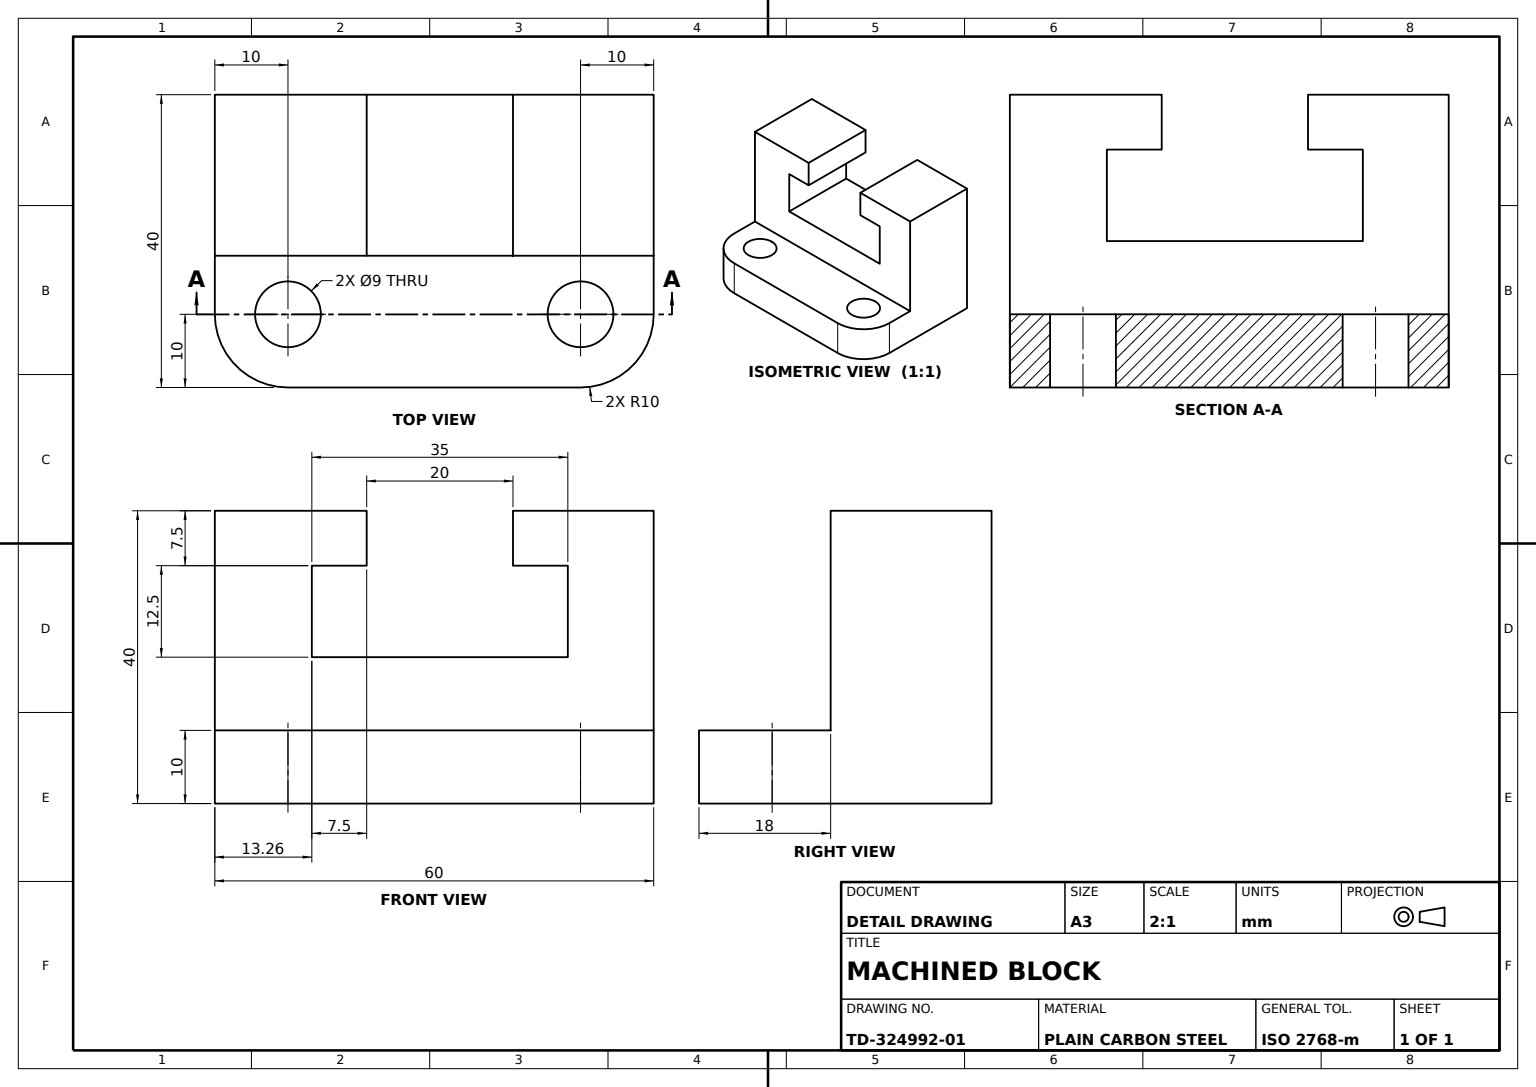
from build123d import *

# Parameters (mm, degrees)
U_BRACKET_BODY_DEPTH      = 22
BASE_PLATE_DEPTH          = 10
MOUNTING_HOLES_SKETCH_R   = 4.5
MOUNTING_HOLES_2X_9_DEPTH = 79.102496759


with BuildPart() as part:
    # U-Bracket Profile Sketch → U-Bracket Body (new body)
    with BuildSketch(Plane.XY):
        Polygon((0, 0), (60, 0), (60, 40), (40.761904762, 40), (40.761904762, 32.5), (48.261904762, 32.5), (48.261904762, 20), (13.261904762, 20), (13.261904762, 32.5), (20.761904762, 32.5), (20.761904762, 40), (0, 40), align=None)
    extrude(amount=U_BRACKET_BODY_DEPTH)

    # Base Plate Sketch → Base Plate (add)
    with BuildSketch(Plane.XZ):
        with BuildLine():
            Line((0, 22), (0, 30))
            ThreePointArc((0, 30), (2.928932188, 37.071067812), (10, 40))
            Line((10, 40), (50, 40))
            ThreePointArc((50, 40), (57.071067812, 37.071067812), (60, 30))
            Line((60, 30), (60, 22))
            Line((60, 22), (60, 0))
            Line((60, 0), (0, 0))
            Line((0, 0), (0, 22))
        make_face()
    extrude(amount=-BASE_PLATE_DEPTH)

    # Mounting Holes Sketch → Mounting Holes 2xØ9 (cut, through all)
    with BuildSketch(Plane(origin=(0, 10, 0), x_dir=(1, 0, 0), z_dir=(0, 1, 0))):
        with Locations(Location((10, -30, 0), (0, 0, 270))):
            Circle(MOUNTING_HOLES_SKETCH_R)
        with Locations(Location((50, -30, 0), (0, 0, 270))):
            Circle(MOUNTING_HOLES_SKETCH_R)
    extrude(amount=-MOUNTING_HOLES_2X_9_DEPTH, mode=Mode.SUBTRACT)


solid = part.part
